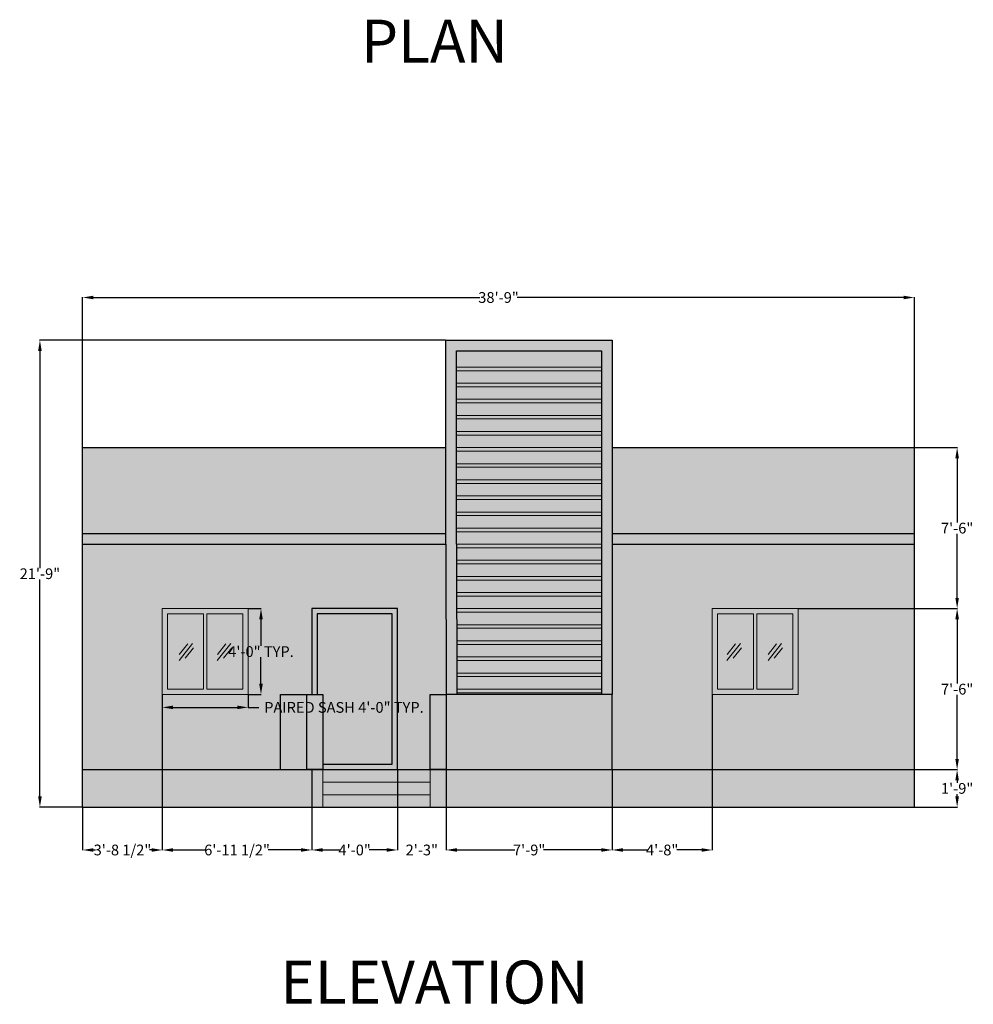
# Model space of a CAD drawing. Units: inches. Extents: x 1966 to 4198, y 2607 to 3884.
# Tile 1 of 8: x 2025 to 2558, y 2607 to 3158. Entities that reach past the tile are written whole.
import ezdxf

# ---------------------------------------------------------------- set-up
doc = ezdxf.new("R2010")
doc.units = ezdxf.units.IN
doc.header["$MEASUREMENT"] = 0
for name, color, linetype, lineweight in [('A-ANNO-TEXT', 4, 'Continuous', 25), ('A-DOOR-PATT', 46, 'Continuous', 13), ('A-ELEV', 7, 'Continuous', 25), ('A-ELEV-PATT', 253, 'Continuous', 13), ('A-ELEV-SCRN', 7, 'Continuous', 18), ('A-ELEV-SCRN-PATT', 18, 'Continuous', 13), ('A-FLOR-STRS', 7, 'Continuous', 18), ('A-GLAZ', 4, 'Continuous', 18), ('A-GLAZ-FRAM-PATT', 32, 'Continuous', 13), ('A-GLAZ-PATT', 14, 'Continuous', 13), ('dimension', 90, 'Continuous', 18), ('door', 17, 'Continuous', 25)]:
    doc.layers.add(name, color=color, linetype=linetype, lineweight=lineweight)
doc.styles.get("Standard").update_dxf_attribs({"font": 'arial.ttf'})
doc.dimstyles.get("Standard").update_dxf_attribs({"dimtxt": 6, "dimasz": 6, "dimexe": 0.18, "dimexo": 0.0625, "dimgap": 0.09, "dimtad": 0, "dimtih": 1, "dimtoh": 1, "dimdec": 1, "dimzin": 0, "dimdsep": 46, "dimlunit": 3, "dimtxsty": 'Standard', "dimcen": 0.09, "dimadec": 0, "dimazin": 0, "dimtfac": 1, "dimtdec": 1, "dimtofl": 0, "dimtmove": 0, "dimatfit": 3, "dimfxl": 1, "dimtolj": 1, "dimtzin": 0, "dimarcsym": 0})

# ---------------------------------------------------------------- blocks, each defined once
blk = doc.blocks.new('SASH-PAIR-ELEV')
for p, q in [((23, 3), (23, 45)), ((25, 3), (25, 45))]:
    blk.add_line(p, q)
blk.add_lwpolyline([(0, 48), (48, 48), (48, 0), (0, 0)], close=True)
for points in [[(23, 3), (3, 3), (3, 45), (23, 45)], [(25, 45), (45, 45), (45, 3), (25, 3)]]:
    blk.add_lwpolyline(points)
blk = doc.blocks.new('GLASS-REFLECTION-MARK')
for p, q in [((0, 0), (7.56, 9.46)), ((0.05, 3.27), (4.8, 9.22)), ((3.48, 1.15), (8.1, 6.93))]:
    blk.add_line(p, q)
blk = doc.blocks.new('*D63')
at = {"layer": 'Defpoints', "color": 0, "transparency": 16777216}
for p in [(2104.97, 2780.47), (2152.97, 2780.47), (2152.97, 2773.27)]:
    blk.add_point(p, dxfattribs=at)
at = {"layer": 'dimension', "color": 0, "lineweight": -2, "transparency": 16777216}
for p, q in [((2104.97, 2780.4), (2104.97, 2773.09)), ((2152.97, 2780.4), (2152.97, 2773.09)), ((2110.97, 2773.27), (2146.97, 2773.27)), ((2152.97, 2773.27), (2158.97, 2773.27))]:
    blk.add_line(p, q, dxfattribs=at)
at = {"layer": 'dimension', "color": 0, "transparency": 16777216}
for points in [[(2110.97, 2774.27), (2110.97, 2772.27), (2104.97, 2773.27)], [(2146.97, 2774.27), (2146.97, 2772.27), (2152.97, 2773.27)]]:
    blk.add_solid(points, dxfattribs=at)
at = {"layer": 'dimension', "color": 0, "transparency": 16777216, "insert": (2206.54, 2773.27), "char_height": 6, "attachment_point": 5}
blk.add_mtext('\\A1;PAIRED SASH 4\'-0" TYP.', dxfattribs=at)
blk = doc.blocks.new('*D64')
at = {"layer": 'Defpoints', "color": 0, "transparency": 16777216}
for p in [(2152.97, 2828.47), (2160.17, 2828.47), (2152.97, 2780.47)]:
    blk.add_point(p, dxfattribs=at)
at = {"layer": 'dimension', "color": 0, "lineweight": -2, "transparency": 16777216}
for p, q in [((2153.03, 2828.47), (2160.35, 2828.47)), ((2160.17, 2822.47), (2160.17, 2807.62)), ((2160.17, 2786.47), (2160.17, 2801.31)), ((2153.03, 2780.47), (2160.35, 2780.47))]:
    blk.add_line(p, q, dxfattribs=at)
at = {"layer": 'dimension', "color": 0, "transparency": 16777216}
for points in [[(2159.17, 2822.47), (2161.17, 2822.47), (2160.17, 2828.47)], [(2159.17, 2786.47), (2161.17, 2786.47), (2160.17, 2780.47)]]:
    blk.add_solid(points, dxfattribs=at)
at = {"layer": 'dimension', "color": 0, "transparency": 16777216, "insert": (2160.17, 2804.47), "char_height": 6, "attachment_point": 5}
blk.add_mtext('\\A1;4\'-0" TYP.', dxfattribs=at)
blk = doc.blocks.new('*D85')
at = {"layer": 'Defpoints', "color": 0, "transparency": 16777216}
for p in [(2188.6, 2738.47), (2236.46, 2738.47), (2236.46, 2693.57)]:
    blk.add_point(p, dxfattribs=at)
at = {"layer": 'dimension', "color": 0, "lineweight": -2, "transparency": 16777216}
for p, q in [((2188.6, 2738.4), (2188.6, 2693.39)), ((2236.46, 2738.4), (2236.46, 2693.39)), ((2194.6, 2693.57), (2204.35, 2693.57)), ((2230.46, 2693.57), (2220.72, 2693.57))]:
    blk.add_line(p, q, dxfattribs=at)
at = {"layer": 'dimension', "color": 0, "transparency": 16777216}
for points in [[(2194.6, 2694.57), (2194.6, 2692.57), (2188.6, 2693.57)], [(2230.46, 2694.57), (2230.46, 2692.57), (2236.46, 2693.57)]]:
    blk.add_solid(points, dxfattribs=at)
at = {"layer": 'dimension', "color": 0, "transparency": 16777216, "insert": (2212.53, 2693.57), "char_height": 6, "attachment_point": 5}
blk.add_mtext('\\A1;4\'-0"', dxfattribs=at)
blk = doc.blocks.new('*D102')
at = {"layer": 'Defpoints', "color": 0, "transparency": 16777216}
for p in [(2525.47, 3002.37), (2060.47, 2918.47), (2525.47, 2918.47)]:
    blk.add_point(p, dxfattribs=at)
at = {"layer": 'dimension', "color": 0, "lineweight": -2, "transparency": 16777216}
for p, q in [((2060.47, 2918.53), (2060.47, 3002.55)), ((2066.47, 3002.37), (2282.58, 3002.37)), ((2519.47, 3002.37), (2303.37, 3002.37)), ((2525.47, 2918.53), (2525.47, 3002.55))]:
    blk.add_line(p, q, dxfattribs=at)
at = {"layer": 'dimension', "color": 0, "transparency": 16777216}
for points in [[(2066.47, 3003.37), (2066.47, 3001.37), (2060.47, 3002.37)], [(2519.47, 3003.37), (2519.47, 3001.37), (2525.47, 3002.37)]]:
    blk.add_solid(points, dxfattribs=at)
at = {"layer": 'dimension', "color": 0, "transparency": 16777216, "insert": (2292.97, 3002.37), "char_height": 6, "attachment_point": 5}
blk.add_mtext('\\A1;38\'-9"', dxfattribs=at)
blk = doc.blocks.new('*D103')
at = {"layer": 'Defpoints', "color": 0, "transparency": 16777216}
for p in [(2036.57, 2978.47), (2263.47, 2978.47), (2060.47, 2717.47)]:
    blk.add_point(p, dxfattribs=at)
at = {"layer": 'dimension', "color": 0, "lineweight": -2, "transparency": 16777216}
for p, q in [((2263.41, 2978.47), (2036.39, 2978.47)), ((2036.57, 2972.47), (2036.57, 2851.12)), ((2036.57, 2723.47), (2036.57, 2844.81)), ((2060.41, 2717.47), (2036.39, 2717.47))]:
    blk.add_line(p, q, dxfattribs=at)
at = {"layer": 'dimension', "color": 0, "transparency": 16777216}
for points in [[(2035.57, 2972.47), (2037.57, 2972.47), (2036.57, 2978.47)], [(2035.57, 2723.47), (2037.57, 2723.47), (2036.57, 2717.47)]]:
    blk.add_solid(points, dxfattribs=at)
at = {"layer": 'dimension', "color": 0, "transparency": 16777216, "insert": (2036.57, 2847.97), "char_height": 6, "attachment_point": 5}
blk.add_mtext('\\A1;21\'-9"', dxfattribs=at)
blk = doc.blocks.new('*D104')
at = {"layer": 'Defpoints', "color": 0, "transparency": 16777216}
for p in [(2525.47, 2918.47), (2549.37, 2918.47), (2460.47, 2828.47)]:
    blk.add_point(p, dxfattribs=at)
at = {"layer": 'dimension', "color": 0, "lineweight": -2, "transparency": 16777216}
for p, q in [((2525.54, 2918.47), (2549.55, 2918.47)), ((2549.37, 2912.47), (2549.37, 2876.62)), ((2549.37, 2834.47), (2549.37, 2870.31)), ((2460.54, 2828.47), (2549.55, 2828.47))]:
    blk.add_line(p, q, dxfattribs=at)
at = {"layer": 'dimension', "color": 0, "transparency": 16777216}
for points in [[(2548.37, 2912.47), (2550.37, 2912.47), (2549.37, 2918.47)], [(2548.37, 2834.47), (2550.37, 2834.47), (2549.37, 2828.47)]]:
    blk.add_solid(points, dxfattribs=at)
at = {"layer": 'dimension', "color": 0, "transparency": 16777216, "insert": (2549.37, 2873.47), "char_height": 6, "attachment_point": 5}
blk.add_mtext('\\A1;7\'-6"', dxfattribs=at)
blk = doc.blocks.new('*D105')
at = {"layer": 'Defpoints', "color": 0, "transparency": 16777216}
for p in [(2104.97, 2780.47), (2060.47, 2717.47), (2104.97, 2693.57)]:
    blk.add_point(p, dxfattribs=at)
at = {"layer": 'dimension', "color": 0, "lineweight": -2, "transparency": 16777216}
for p, q in [((2104.97, 2780.4), (2104.97, 2693.39)), ((2060.47, 2717.4), (2060.47, 2693.39)), ((2066.47, 2693.57), (2067.67, 2693.57)), ((2098.97, 2693.57), (2097.78, 2693.57))]:
    blk.add_line(p, q, dxfattribs=at)
at = {"layer": 'dimension', "color": 0, "transparency": 16777216}
for points in [[(2066.47, 2694.57), (2066.47, 2692.57), (2060.47, 2693.57)], [(2098.97, 2694.57), (2098.97, 2692.57), (2104.97, 2693.57)]]:
    blk.add_solid(points, dxfattribs=at)
at = {"layer": 'dimension', "color": 0, "transparency": 16777216, "insert": (2082.72, 2693.57), "char_height": 6, "attachment_point": 5}
blk.add_mtext('\\A1;3\'-8 1/2"', dxfattribs=at)
blk = doc.blocks.new('*D106')
at = {"layer": 'Defpoints', "color": 0, "transparency": 16777216}
for p in [(2104.97, 2780.47), (2188.6, 2738.47), (2188.6, 2693.57)]:
    blk.add_point(p, dxfattribs=at)
at = {"layer": 'dimension', "color": 0, "lineweight": -2, "transparency": 16777216}
for p, q in [((2104.97, 2780.4), (2104.97, 2693.39)), ((2188.6, 2738.4), (2188.6, 2693.39)), ((2110.97, 2693.57), (2129.38, 2693.57)), ((2182.6, 2693.57), (2164.19, 2693.57))]:
    blk.add_line(p, q, dxfattribs=at)
at = {"layer": 'dimension', "color": 0, "transparency": 16777216}
for points in [[(2110.97, 2694.57), (2110.97, 2692.57), (2104.97, 2693.57)], [(2182.6, 2694.57), (2182.6, 2692.57), (2188.6, 2693.57)]]:
    blk.add_solid(points, dxfattribs=at)
at = {"layer": 'dimension', "color": 0, "transparency": 16777216, "insert": (2146.78, 2693.57), "char_height": 6, "attachment_point": 5}
blk.add_mtext('\\A1;6\'-11 1/2"', dxfattribs=at)
blk = doc.blocks.new('*D107')
at = {"layer": 'Defpoints', "color": 0, "transparency": 16777216}
for p in [(2236.46, 2738.47), (2263.7, 2738.47), (2263.7, 2693.57)]:
    blk.add_point(p, dxfattribs=at)
at = {"layer": 'dimension', "color": 0, "lineweight": -2, "transparency": 16777216}
for p, q in [((2236.46, 2738.4), (2236.46, 2693.39)), ((2263.7, 2738.4), (2263.7, 2693.39)), ((2230.46, 2693.57), (2224.46, 2693.57)), ((2269.7, 2693.57), (2275.7, 2693.57))]:
    blk.add_line(p, q, dxfattribs=at)
at = {"layer": 'dimension', "color": 0, "transparency": 16777216}
for points in [[(2230.46, 2694.57), (2230.46, 2692.57), (2236.46, 2693.57)], [(2269.7, 2694.57), (2269.7, 2692.57), (2263.7, 2693.57)]]:
    blk.add_solid(points, dxfattribs=at)
at = {"layer": 'dimension', "color": 0, "transparency": 16777216, "insert": (2250.08, 2693.57), "char_height": 6, "attachment_point": 5}
blk.add_mtext('\\A1;2\'-3"', dxfattribs=at)
blk = doc.blocks.new('*D108')
at = {"layer": 'Defpoints', "color": 0, "transparency": 16777216}
for p in [(2263.7, 2738.47), (2356.47, 2738.47), (2356.47, 2693.57)]:
    blk.add_point(p, dxfattribs=at)
at = {"layer": 'dimension', "color": 0, "lineweight": -2, "transparency": 16777216}
for p, q in [((2263.7, 2738.4), (2263.7, 2693.39)), ((2356.47, 2738.4), (2356.47, 2693.39)), ((2269.7, 2693.57), (2302.05, 2693.57)), ((2350.47, 2693.57), (2318.13, 2693.57))]:
    blk.add_line(p, q, dxfattribs=at)
at = {"layer": 'dimension', "color": 0, "transparency": 16777216}
for points in [[(2269.7, 2694.57), (2269.7, 2692.57), (2263.7, 2693.57)], [(2350.47, 2694.57), (2350.47, 2692.57), (2356.47, 2693.57)]]:
    blk.add_solid(points, dxfattribs=at)
at = {"layer": 'dimension', "color": 0, "transparency": 16777216, "insert": (2310.09, 2693.57), "char_height": 6, "attachment_point": 5}
blk.add_mtext('\\A1;7\'-9"', dxfattribs=at)
blk = doc.blocks.new('*D109')
at = {"layer": 'Defpoints', "color": 0, "transparency": 16777216}
for p in [(2412.47, 2780.47), (2356.47, 2738.47), (2412.47, 2693.57)]:
    blk.add_point(p, dxfattribs=at)
at = {"layer": 'dimension', "color": 0, "lineweight": -2, "transparency": 16777216}
for p, q in [((2412.47, 2780.4), (2412.47, 2693.39)), ((2356.47, 2738.4), (2356.47, 2693.39)), ((2362.47, 2693.57), (2376.29, 2693.57)), ((2406.47, 2693.57), (2392.66, 2693.57))]:
    blk.add_line(p, q, dxfattribs=at)
at = {"layer": 'dimension', "color": 0, "transparency": 16777216}
for points in [[(2362.47, 2694.57), (2362.47, 2692.57), (2356.47, 2693.57)], [(2406.47, 2694.57), (2406.47, 2692.57), (2412.47, 2693.57)]]:
    blk.add_solid(points, dxfattribs=at)
at = {"layer": 'dimension', "color": 0, "transparency": 16777216, "insert": (2384.47, 2693.57), "char_height": 6, "attachment_point": 5}
blk.add_mtext('\\A1;4\'-8"', dxfattribs=at)
blk = doc.blocks.new('*D110')
at = {"layer": 'Defpoints', "color": 0, "transparency": 16777216}
for p in [(2460.47, 2828.47), (2525.47, 2738.47), (2549.37, 2738.47)]:
    blk.add_point(p, dxfattribs=at)
at = {"layer": 'dimension', "color": 0, "lineweight": -2, "transparency": 16777216}
for p, q in [((2460.54, 2828.47), (2549.55, 2828.47)), ((2549.37, 2822.47), (2549.37, 2786.62)), ((2549.37, 2744.47), (2549.37, 2780.31)), ((2525.54, 2738.47), (2549.55, 2738.47))]:
    blk.add_line(p, q, dxfattribs=at)
at = {"layer": 'dimension', "color": 0, "transparency": 16777216}
for points in [[(2548.37, 2822.47), (2550.37, 2822.47), (2549.37, 2828.47)], [(2548.37, 2744.47), (2550.37, 2744.47), (2549.37, 2738.47)]]:
    blk.add_solid(points, dxfattribs=at)
at = {"layer": 'dimension', "color": 0, "transparency": 16777216, "insert": (2549.37, 2783.47), "char_height": 6, "attachment_point": 5}
blk.add_mtext('\\A1;7\'-6"', dxfattribs=at)
blk = doc.blocks.new('*D111')
at = {"layer": 'Defpoints', "color": 0, "transparency": 16777216}
for p in [(2525.47, 2738.47), (2525.47, 2717.47), (2549.37, 2717.47)]:
    blk.add_point(p, dxfattribs=at)
at = {"layer": 'dimension', "color": 0, "lineweight": -2, "transparency": 16777216}
for p, q in [((2525.54, 2738.47), (2549.55, 2738.47)), ((2549.37, 2732.47), (2549.37, 2731.12)), ((2549.37, 2723.47), (2549.37, 2724.81)), ((2525.54, 2717.47), (2549.55, 2717.47))]:
    blk.add_line(p, q, dxfattribs=at)
at = {"layer": 'dimension', "color": 0, "transparency": 16777216}
for points in [[(2548.37, 2732.47), (2550.37, 2732.47), (2549.37, 2738.47)], [(2548.37, 2723.47), (2550.37, 2723.47), (2549.37, 2717.47)]]:
    blk.add_solid(points, dxfattribs=at)
at = {"layer": 'dimension', "color": 0, "transparency": 16777216, "insert": (2549.37, 2727.97), "char_height": 6, "attachment_point": 5}
blk.add_mtext('\\A1;1\'-9"', dxfattribs=at)

msp = doc.modelspace()

# ---------------------------------------------------------------- hatches: boundary and pattern name
at = {"layer": 'A-DOOR-PATT', "transparency": 33554577}
h = msp.add_hatch(color=256, dxfattribs=at)
h.dxf.hatch_style = 1
h.paths.add_polyline_path([(2188.6, 2780.47), (2191.6, 2780.47), (2191.6, 2825.47), (2233.46, 2825.47), (2233.46, 2741.47), (2194.7, 2741.47), (2194.7, 2738.47), (2236.46, 2738.47), (2236.46, 2828.47), (2188.6, 2828.47)])
at = {"layer": 'A-DOOR-PATT', "transparency": 33554653}
h = msp.add_hatch(color=256, dxfattribs=at)
h.dxf.hatch_style = 1
h.paths.add_polyline_path([(2233.46, 2825.47), (2191.6, 2825.47), (2191.6, 2780.47), (2194.7, 2780.47), (2194.7, 2741.47), (2233.46, 2741.47)])
at = {"layer": 'A-ELEV-PATT', "transparency": 33554577}
h = msp.add_hatch(color=256, dxfattribs=at)
h.dxf.hatch_style = 1
h.paths.add_polyline_path([(2350.47, 2972.47), (2350.47, 2864.47), (2350.47, 2780.47), (2356.47, 2780.47), (2356.47, 2864.47), (2356.47, 2978.47), (2263.47, 2978.47), (2263.47, 2864.47), (2263.7, 2780.47), (2269.7, 2780.47), (2269.47, 2864.47), (2269.47, 2864.47), (2269.47, 2972.47)])
h = msp.add_hatch(color=256, dxfattribs=at)
h.dxf.hatch_style = 1
h.paths.add_polyline_path([(2350.47, 2963.47), (2350.47, 2972.47), (2269.47, 2972.47), (2269.47, 2963.47)])
h.paths.add_polyline_path([(2269.47, 2961.47), (2269.47, 2954.47), (2350.47, 2954.47), (2350.47, 2961.47)])
h.paths.add_polyline_path([(2350.47, 2945.47), (2350.47, 2952.47), (2269.47, 2952.47), (2269.47, 2945.47)])
h.paths.add_polyline_path([(2350.47, 2936.47), (2350.47, 2943.47), (2269.47, 2943.47), (2269.47, 2936.47)])
h.paths.add_polyline_path([(2269.47, 2934.47), (2269.47, 2927.47), (2350.47, 2927.47), (2350.47, 2934.47)])
h.paths.add_polyline_path([(2350.47, 2918.47), (2350.47, 2925.47), (2269.47, 2925.47), (2269.47, 2918.47)])
h.paths.add_polyline_path([(2350.47, 2909.47), (2350.47, 2916.47), (2269.47, 2916.47), (2269.47, 2909.47)])
h.paths.add_polyline_path([(2350.47, 2900.47), (2350.47, 2907.47), (2269.47, 2907.47), (2269.47, 2900.47)])
h.paths.add_polyline_path([(2350.47, 2891.47), (2350.47, 2898.47), (2269.47, 2898.47), (2269.47, 2891.47)])
h.paths.add_polyline_path([(2269.47, 2889.47), (2269.47, 2882.47), (2350.47, 2882.47), (2350.47, 2889.47)])
h.paths.add_polyline_path([(2269.47, 2880.47), (2269.47, 2873.47), (2350.47, 2873.47), (2350.47, 2880.47)])
h.paths.add_polyline_path([(2350.47, 2864.47), (2350.47, 2871.47), (2269.47, 2871.47), (2269.47, 2864.47), (2269.47, 2864.47)])
h.paths.add_polyline_path([(2350.47, 2855.47), (2350.47, 2862.47), (2269.48, 2862.47), (2269.5, 2855.47)])
h.paths.add_polyline_path([(2269.5, 2853.47), (2269.52, 2846.47), (2350.47, 2846.47), (2350.47, 2853.47)])
h.paths.add_polyline_path([(2350.47, 2837.47), (2350.47, 2844.47), (2269.53, 2844.47), (2269.55, 2837.47)])
h.paths.add_polyline_path([(2350.47, 2828.47), (2350.47, 2835.47), (2269.55, 2835.47), (2269.57, 2828.47)])
h.paths.add_polyline_path([(2350.47, 2819.47), (2350.47, 2826.47), (2269.58, 2826.47), (2269.6, 2819.47)])
h.paths.add_polyline_path([(2350.47, 2810.47), (2350.47, 2817.47), (2269.6, 2817.47), (2269.62, 2810.47)])
h.paths.add_polyline_path([(2350.47, 2801.47), (2350.47, 2808.47), (2269.63, 2808.47), (2269.64, 2801.47)])
h.paths.add_polyline_path([(2269.65, 2799.47), (2269.67, 2792.47), (2350.47, 2792.47), (2350.47, 2799.47)])
h.paths.add_polyline_path([(2269.67, 2790.47), (2269.69, 2783.47), (2350.47, 2783.47), (2350.47, 2790.47)])
h.paths.add_polyline_path([(2350.47, 2780.47), (2350.47, 2781.47), (2269.7, 2781.47), (2269.7, 2780.47)])
h = msp.add_hatch(color=256, dxfattribs=at)
h.dxf.hatch_style = 1
h.paths.add_polyline_path([(2356.47, 2918.47), (2356.47, 2870.47), (2525.47, 2870.47), (2525.47, 2918.47)])
h.paths.add_polyline_path([(2263.47, 2870.47), (2263.47, 2918.47), (2060.47, 2918.47), (2060.47, 2870.47)])
at = {"layer": 'A-ELEV-PATT', "transparency": 33554630}
h = msp.add_hatch(color=256, dxfattribs=at)
h.dxf.hatch_style = 1
h.paths.add_polyline_path([(2263.47, 2864.47), (2263.47, 2870.47), (2060.47, 2870.47), (2060.47, 2864.47)])
h.paths.add_polyline_path([(2356.47, 2870.47), (2356.47, 2864.47), (2525.47, 2864.47), (2525.47, 2870.47)])
at = {"layer": 'A-ELEV-PATT'}
h = msp.add_hatch(color=256, dxfattribs=at)
h.dxf.hatch_style = 1
h.paths.add_polyline_path([(2060.47, 2864.47), (2060.47, 2738.47), (2171.06, 2738.47), (2171.06, 2780.47), (2185.7, 2780.47), (2188.6, 2780.47), (2188.6, 2828.47), (2236.46, 2828.47), (2236.46, 2738.47), (2254.7, 2738.47), (2254.7, 2780.47), (2263.7, 2780.47), (2263.47, 2864.47)])
h.paths.add_polyline_path([(2152.97, 2828.47), (2152.97, 2780.47), (2104.97, 2780.47), (2104.97, 2828.47)], flags=16)
h.paths.add_polyline_path([(2149.97, 2825.47), (2149.97, 2783.47), (2129.97, 2783.47), (2129.97, 2825.47)], flags=0)
h.paths.add_polyline_path([(2127.97, 2825.47), (2127.97, 2783.47), (2107.97, 2783.47), (2107.97, 2825.47)], flags=0)
h.paths.add_polyline_path([(2356.47, 2780.47), (2356.47, 2738.47), (2525.47, 2738.47), (2525.47, 2864.47), (2356.47, 2864.47)])
h.paths.add_polyline_path([(2412.47, 2828.47), (2460.47, 2828.47), (2460.47, 2780.47), (2412.47, 2780.47)], flags=16)
h.paths.add_polyline_path([(2415.47, 2825.47), (2435.47, 2825.47), (2435.47, 2783.47), (2415.47, 2783.47)], flags=0)
h.paths.add_polyline_path([(2437.47, 2825.47), (2457.47, 2825.47), (2457.47, 2783.47), (2437.47, 2783.47)], flags=0)
h = msp.add_hatch(color=256, dxfattribs=at)
h.dxf.hatch_style = 1
h.paths.add_polyline_path([(2185.7, 2780.47), (2171.06, 2780.47), (2171.06, 2738.47), (2185.7, 2738.47)])
h.paths.add_polyline_path([(2356.47, 2780.47), (2263.7, 2780.47), (2263.7, 2738.47), (2356.47, 2738.47)])
h = msp.add_hatch(color=256, dxfattribs=at)
h.dxf.hatch_style = 1
h.paths.add_polyline_path([(2185.7, 2738.47), (2194.7, 2738.47), (2194.7, 2780.47), (2185.7, 2780.47)])
h.paths.add_polyline_path([(2263.7, 2780.47), (2254.7, 2780.47), (2254.7, 2738.47), (2263.7, 2738.47)])
at = {"layer": 'A-ELEV-PATT', "transparency": 33554577}
h = msp.add_hatch(color=256, dxfattribs=at)
h.dxf.hatch_style = 1
h.paths.add_polyline_path([(2194.7, 2717.47), (2194.7, 2738.47), (2185.7, 2738.47), (2060.47, 2738.47), (2060.47, 2717.47)])
h.paths.add_polyline_path([(2525.47, 2717.47), (2525.47, 2738.47), (2254.7, 2738.47), (2254.7, 2717.47)])
h = msp.add_hatch(color=256, dxfattribs=at)
h.dxf.hatch_style = 1
h.paths.add_polyline_path([(2254.7, 2738.47), (2194.7, 2738.47), (2194.7, 2731.47), (2254.7, 2731.47)])
h.paths.add_polyline_path([(2254.7, 2731.47), (2194.7, 2731.47), (2194.7, 2724.47), (2254.7, 2724.47)])
h.paths.add_polyline_path([(2254.7, 2724.47), (2194.7, 2724.47), (2194.7, 2717.47), (2254.7, 2717.47)])
at = {"layer": 'A-ELEV-SCRN-PATT', "transparency": 33554577}
h = msp.add_hatch(color=256, dxfattribs=at)
h.dxf.hatch_style = 1
h.paths.add_polyline_path([(2350.47, 2963.47), (2269.47, 2963.47), (2269.47, 2961.47), (2350.47, 2961.47)])
h.paths.add_polyline_path([(2350.47, 2954.47), (2269.47, 2954.47), (2269.47, 2952.47), (2350.47, 2952.47)])
h.paths.add_polyline_path([(2350.47, 2945.47), (2269.47, 2945.47), (2269.47, 2943.47), (2350.47, 2943.47)])
h.paths.add_polyline_path([(2350.47, 2936.47), (2269.47, 2936.47), (2269.47, 2934.47), (2350.47, 2934.47)])
h.paths.add_polyline_path([(2350.47, 2927.47), (2269.47, 2927.47), (2269.47, 2925.47), (2350.47, 2925.47)])
h.paths.add_polyline_path([(2350.47, 2918.47), (2269.47, 2918.47), (2269.47, 2916.47), (2350.47, 2916.47)])
h.paths.add_polyline_path([(2350.47, 2909.47), (2269.47, 2909.47), (2269.47, 2907.47), (2350.47, 2907.47)])
h.paths.add_polyline_path([(2350.47, 2900.47), (2269.47, 2900.47), (2269.47, 2898.47), (2350.47, 2898.47)])
h.paths.add_polyline_path([(2350.47, 2891.47), (2269.47, 2891.47), (2269.47, 2889.47), (2350.47, 2889.47)])
h.paths.add_polyline_path([(2350.47, 2882.47), (2269.47, 2882.47), (2269.47, 2880.47), (2350.47, 2880.47)])
h.paths.add_polyline_path([(2350.47, 2873.47), (2269.47, 2873.47), (2269.47, 2871.47), (2350.47, 2871.47)])
h.paths.add_polyline_path([(2350.47, 2864.47), (2269.47, 2864.47), (2269.48, 2862.47), (2350.47, 2862.47)])
h.paths.add_polyline_path([(2350.47, 2855.47), (2269.5, 2855.47), (2269.5, 2853.47), (2350.47, 2853.47)])
h.paths.add_polyline_path([(2350.47, 2846.47), (2269.52, 2846.47), (2269.53, 2844.47), (2350.47, 2844.47)])
h.paths.add_polyline_path([(2350.47, 2837.47), (2269.55, 2837.47), (2269.55, 2835.47), (2350.47, 2835.47)])
h.paths.add_polyline_path([(2350.47, 2828.47), (2269.57, 2828.47), (2269.58, 2826.47), (2350.47, 2826.47)])
h.paths.add_polyline_path([(2350.47, 2819.47), (2269.6, 2819.47), (2269.6, 2817.47), (2350.47, 2817.47)])
h.paths.add_polyline_path([(2350.47, 2810.47), (2269.62, 2810.47), (2269.63, 2808.47), (2350.47, 2808.47)])
h.paths.add_polyline_path([(2350.47, 2801.47), (2269.64, 2801.47), (2269.65, 2799.47), (2350.47, 2799.47)])
h.paths.add_polyline_path([(2350.47, 2792.47), (2269.67, 2792.47), (2269.67, 2790.47), (2350.47, 2790.47)])
h.paths.add_polyline_path([(2350.47, 2783.47), (2269.69, 2783.47), (2269.7, 2781.47), (2350.47, 2781.47)])
at = {"layer": 'A-GLAZ-FRAM-PATT'}
h = msp.add_hatch(color=256, dxfattribs=at)
h.dxf.hatch_style = 1
h.paths.add_polyline_path([(2152.97, 2780.47), (2152.97, 2828.47), (2104.97, 2828.47), (2104.97, 2780.47)])
h.paths.add_polyline_path([(2129.97, 2783.47), (2129.97, 2825.47), (2149.97, 2825.47), (2149.97, 2783.47)], flags=16)
h.paths.add_polyline_path([(2127.97, 2783.47), (2107.97, 2783.47), (2107.97, 2825.47), (2127.97, 2825.47)], flags=16)
h.paths.add_polyline_path([(2460.47, 2780.47), (2460.47, 2828.47), (2412.47, 2828.47), (2412.47, 2780.47)])
h.paths.add_polyline_path([(2435.47, 2783.47), (2415.47, 2783.47), (2415.47, 2825.47), (2435.47, 2825.47)], flags=16)
h.paths.add_polyline_path([(2437.47, 2783.47), (2437.47, 2825.47), (2457.47, 2825.47), (2457.47, 2783.47)], flags=16)
at = {"layer": 'A-GLAZ-PATT', "transparency": 33554508}
h = msp.add_hatch(color=256, dxfattribs=at)
h.dxf.hatch_style = 1
h.paths.add_polyline_path([(2107.97, 2825.47), (2107.97, 2783.47), (2127.97, 2783.47), (2127.97, 2825.47)])
h.paths.add_polyline_path([(2129.97, 2825.47), (2129.97, 2783.47), (2149.97, 2783.47), (2149.97, 2825.47)])
h.paths.add_polyline_path([(2415.47, 2825.47), (2415.47, 2783.47), (2435.47, 2783.47), (2435.47, 2825.47)])
h.paths.add_polyline_path([(2437.47, 2825.47), (2437.47, 2783.47), (2457.47, 2783.47), (2457.47, 2825.47)])

# ---------------------------------------------------------------- linework, layer by layer
at = {"layer": 'A-ELEV'}
for p, q in [((2263.47, 2864.47), (2263.47, 2978.47)), ((2263.47, 2978.47), (2356.47, 2978.47)), ((2356.47, 2978.47), (2356.47, 2864.47)), ((2269.47, 2864.47), (2269.47, 2972.47)), ((2269.47, 2972.47), (2350.47, 2972.47)), ((2350.47, 2972.47), (2350.47, 2864.47)), ((2060.47, 2717.47), (2060.47, 2918.47)), ((2060.47, 2918.47), (2263.47, 2918.47)), ((2356.47, 2918.47), (2525.47, 2918.47)), ((2525.47, 2717.47), (2525.47, 2918.47)), ((2060.47, 2870.47), (2263.47, 2870.47)), ((2356.47, 2870.47), (2525.47, 2870.47)), ((2060.47, 2864.47), (2263.47, 2864.47)), ((2263.47, 2864.47), (2263.7, 2780.47)), ((2269.47, 2864.48), (2269.7, 2780.48)), ((2350.47, 2864.47), (2350.47, 2780.47)), ((2356.47, 2864.47), (2356.47, 2780.47)), ((2356.47, 2864.47), (2525.47, 2864.47)), ((2171.06, 2738.47), (2171.06, 2780.47)), ((2171.06, 2780.47), (2185.7, 2780.47)), ((2171.06, 2780.47), (2194.7, 2780.47)), ((2185.7, 2780.47), (2185.7, 2738.47)), ((2185.7, 2780.47), (2194.7, 2780.47)), ((2194.7, 2780.47), (2194.7, 2738.47)), ((2254.7, 2738.47), (2254.7, 2780.47)), ((2254.7, 2780.47), (2263.7, 2780.47)), ((2263.7, 2780.47), (2263.7, 2738.47)), ((2356.47, 2780.47), (2263.7, 2780.47)), ((2356.47, 2738.47), (2356.47, 2780.47)), ((2060.47, 2738.47), (2525.47, 2738.47)), ((2194.7, 2738.47), (2185.7, 2738.47)), ((2194.7, 2738.47), (2254.7, 2738.47)), ((2263.7, 2738.47), (2254.7, 2738.47)), ((2254.7, 2738.47), (2356.47, 2738.47)), ((2060.47, 2717.47), (2525.47, 2717.47))]:
    msp.add_line(p, q, dxfattribs=at)
at = {"layer": 'A-ELEV-SCRN'}
for p, q in [((2269.47, 2963.47), (2350.47, 2963.47)), ((2269.47, 2961.47), (2350.47, 2961.47)), ((2269.47, 2954.47), (2350.47, 2954.47)), ((2269.47, 2952.47), (2350.47, 2952.47)), ((2269.47, 2945.47), (2350.47, 2945.47)), ((2269.47, 2943.47), (2350.47, 2943.47)), ((2269.47, 2936.47), (2350.47, 2936.47)), ((2269.47, 2934.47), (2350.47, 2934.47)), ((2269.47, 2927.47), (2350.47, 2927.47)), ((2269.47, 2925.47), (2350.47, 2925.47)), ((2269.47, 2918.47), (2350.47, 2918.47)), ((2269.47, 2916.47), (2350.47, 2916.47)), ((2269.47, 2909.47), (2350.47, 2909.47)), ((2269.47, 2907.47), (2350.47, 2907.47)), ((2269.47, 2900.47), (2350.47, 2900.47)), ((2269.47, 2898.47), (2350.47, 2898.47)), ((2269.47, 2891.47), (2350.47, 2891.47)), ((2269.47, 2889.47), (2350.47, 2889.47)), ((2269.47, 2882.47), (2350.47, 2882.47)), ((2269.47, 2880.47), (2350.47, 2880.47)), ((2269.47, 2873.47), (2350.47, 2873.47)), ((2269.47, 2871.47), (2350.47, 2871.47)), ((2269.47, 2864.47), (2350.47, 2864.47)), ((2269.47, 2862.47), (2350.47, 2862.47)), ((2269.47, 2853.47), (2350.47, 2853.47)), ((2269.5, 2855.47), (2350.47, 2855.47)), ((2269.52, 2846.47), (2350.47, 2846.47)), ((2269.53, 2844.47), (2350.47, 2844.47)), ((2269.55, 2837.47), (2350.47, 2837.47)), ((2269.55, 2835.47), (2350.47, 2835.47)), ((2269.57, 2828.47), (2350.47, 2828.47)), ((2269.58, 2826.47), (2350.47, 2826.47)), ((2269.6, 2819.47), (2350.47, 2819.47)), ((2269.6, 2817.47), (2350.47, 2817.47)), ((2269.62, 2810.47), (2350.47, 2810.47)), ((2269.63, 2808.47), (2350.47, 2808.47)), ((2269.64, 2801.47), (2350.47, 2801.47)), ((2269.65, 2799.47), (2350.47, 2799.47)), ((2269.67, 2792.47), (2350.47, 2792.47)), ((2269.67, 2790.47), (2350.47, 2790.47)), ((2269.69, 2783.47), (2350.47, 2783.47)), ((2269.7, 2781.47), (2350.47, 2781.47))]:
    msp.add_line(p, q, dxfattribs=at)
at = {"layer": 'A-FLOR-STRS'}
for p, q in [((2194.7, 2738.47), (2194.7, 2717.47)), ((2254.7, 2738.47), (2254.7, 2717.47)), ((2194.7, 2731.47), (2254.7, 2731.47)), ((2194.7, 2724.47), (2254.7, 2724.47))]:
    msp.add_line(p, q, dxfattribs=at)
at = {"layer": 'A-GLAZ'}
msp.add_line((2104.97, 2780.47), (2152.97, 2780.47), dxfattribs=at)
at = {"layer": 'door'}
for points in [[(2188.6, 2738.47), (2236.46, 2738.47), (2236.46, 2828.47), (2188.6, 2828.47), (2188.6, 2780.47)], [(2194.7, 2741.47), (2233.46, 2741.47), (2233.46, 2825.47), (2191.6, 2825.47), (2191.6, 2780.47)]]:
    msp.add_lwpolyline(points, dxfattribs=at)

# ---------------------------------------------------------------- block references
at = {"layer": 'A-GLAZ'}
for name, p in [('SASH-PAIR-ELEV', (2104.97, 2780.47)), ('SASH-PAIR-ELEV', (2412.47, 2780.47)), ('GLASS-REFLECTION-MARK', (2114.39, 2799.56)), ('GLASS-REFLECTION-MARK', (2135.73, 2799.56)), ('GLASS-REFLECTION-MARK', (2420.68, 2799.56)), ('GLASS-REFLECTION-MARK', (2443.65, 2799.56))]:
    msp.add_blockref(name, p, dxfattribs=at)

# ---------------------------------------------------------------- texts
at = {"layer": 'A-ANNO-TEXT', "char_height": 24, "attachment_point": 2}
for s, insert in [('PLAN', (2257.15, 3157.64)), ('ELEVATION', (2257.15, 2631.74))]:
    msp.add_mtext_dynamic_manual_height_columns(s, width=89.9452, gutter_width=1, heights=[0], dxfattribs=dict(at, insert=insert))

# ---------------------------------------------------------------- dimensions: what is measured, and where the dimension line sits
at = {"layer": 'dimension'}
for base, p1, p2, picture, middle in [((2525.47, 3002.37), (2060.47, 2918.47), (2525.47, 2918.47), '*D102', (2292.97, 3002.37)), ((2104.97, 2693.57), (2060.47, 2717.47), (2104.97, 2780.47), '*D105', (2082.72, 2693.57)), ((2188.6, 2693.57), (2104.97, 2780.47), (2188.6, 2738.47), '*D106', (2146.78, 2693.57)), ((2412.47, 2693.57), (2356.47, 2738.47), (2412.47, 2780.47), '*D109', (2384.47, 2693.57)), ((2236.46, 2693.57), (2188.6, 2738.47), (2236.46, 2738.47), '*D85', (2212.53, 2693.57)), ((2263.7, 2693.57), (2236.46, 2738.47), (2263.7, 2738.47), '*D107', (2250.08, 2693.57)), ((2356.47, 2693.57), (2263.7, 2738.47), (2356.47, 2738.47), '*D108', (2310.09, 2693.57))]:
    dim = msp.add_linear_dim(base=base, p1=p1, p2=p2, dimstyle='Standard', override={"dimdec": 1, "dimlfac": 1, "dimrnd": 0, "dimzin": 1, "dimdsep": 46, "dimlunit": 4, "dimfrac": 2}, dxfattribs=at)
    dim.commit()
    dim.dimension.update_dxf_attribs({"geometry": picture, "text_midpoint": middle})
for base, p1, p2, picture, middle in [((2036.57, 2978.47), (2060.47, 2717.47), (2263.47, 2978.47), '*D103', (2036.57, 2847.97)), ((2549.37, 2918.47), (2460.47, 2828.47), (2525.47, 2918.47), '*D104', (2549.37, 2873.47)), ((2549.37, 2738.47), (2460.47, 2828.47), (2525.47, 2738.47), '*D110', (2549.37, 2783.47)), ((2549.37, 2717.47), (2525.47, 2738.47), (2525.47, 2717.47), '*D111', (2549.37, 2727.97))]:
    dim = msp.add_linear_dim(base=base, p1=p1, p2=p2, angle=90, dimstyle='Standard', override={"dimdec": 1, "dimlfac": 1, "dimrnd": 0, "dimzin": 1, "dimdsep": 46, "dimlunit": 4, "dimfrac": 2}, dxfattribs=at)
    dim.commit()
    dim.dimension.update_dxf_attribs({"geometry": picture, "text_midpoint": middle})
dim = msp.add_linear_dim(base=(2160.17, 2828.47), p1=(2152.97, 2780.47), p2=(2152.97, 2828.47), angle=90, text='<> TYP.', dimstyle='Standard', override={"dimdec": 1, "dimlfac": 1, "dimrnd": 0, "dimzin": 1, "dimdsep": 46, "dimlunit": 4, "dimfrac": 2}, dxfattribs=at)
dim.commit()
dim.dimension.update_dxf_attribs({"geometry": '*D64', "text_midpoint": (2160.17, 2804.47)})
dim = msp.add_linear_dim(base=(2152.97, 2773.27), p1=(2104.97, 2780.47), p2=(2152.97, 2780.47), text='PAIRED SASH <> TYP.', dimstyle='Standard', override={"dimdec": 1, "dimlfac": 1, "dimrnd": 0, "dimzin": 1, "dimdsep": 46, "dimlunit": 4, "dimfrac": 2}, dxfattribs=at)
dim.commit()
dim.dimension.update_dxf_attribs({"geometry": '*D63', "text_midpoint": (2206.54, 2773.27)})

doc.saveas('drawing.dxf')
